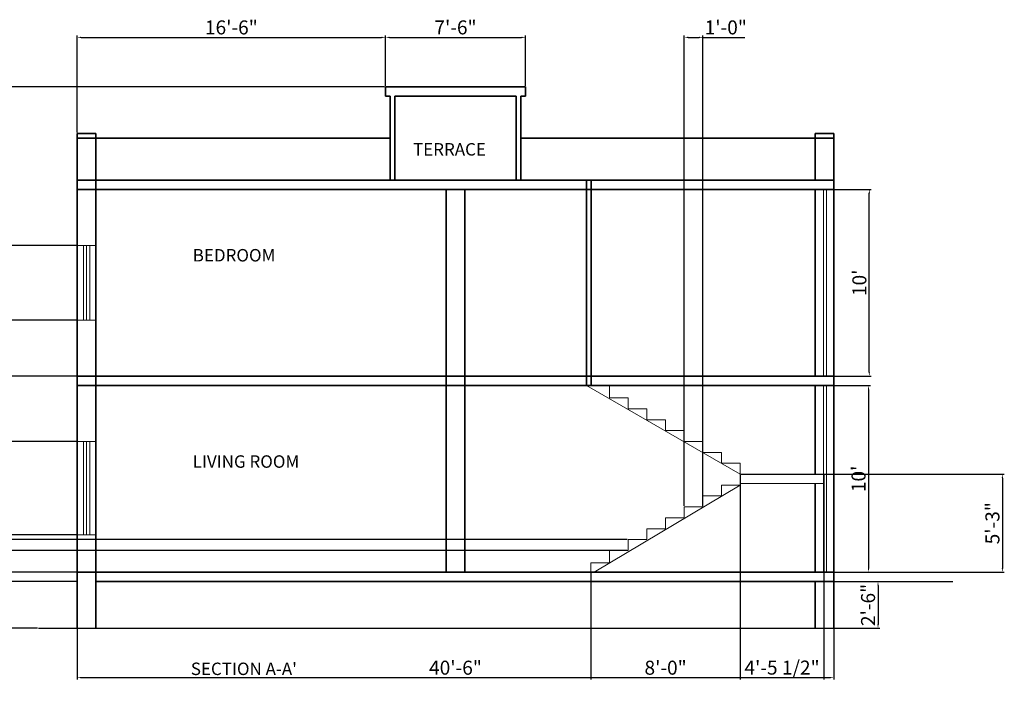
# Model space of a CAD drawing. Units: inches. Extents: x 600 to 1805, y 898 to 2057.
# Tile 4 of 5: x 1172 to 1805, y 898 to 1329. Entities that reach past the tile are written whole.
import ezdxf

# ---------------------------------------------------------------- set-up
doc = ezdxf.new("R2010")
doc.units = ezdxf.units.IN
for name, color, linetype, lineweight in [('A-ANNO-DIMS', 2, 'Continuous', 18), ('A-ANNO-TEXT', 7, 'Continuous', 25), ('A-AREA-IDEN', 7, 'Continuous', 18), ('A-FLOR-STRS', 3, 'Continuous', 20), ('A-SECT', 7, 'Continuous', 35), ('C-SITE', 7, 'Continuous', 25)]:
    doc.layers.add(name, color=color, linetype=linetype, lineweight=lineweight)
doc.layers.add('A-GLAZ', color=244, linetype='Continuous', lineweight=20, true_color=0x991b1e)
doc.styles.get("Standard").update_dxf_attribs({"font": 'arial.ttf'})
doc.dimstyles.new('ISO-25', dxfattribs={"dimtxt": 9, "dimasz": 2.5, "dimexe": 1.25, "dimexo": 0.625, "dimtad": 1, "dimlunit": 3, "dimtxsty": 'Standard', "dimcen": 2.5, "dimadec": 0, "dimazin": 0, "dimtfac": 1, "dimtmove": 0, "dimatfit": 3, "dimfxl": 1, "dimarcsym": 0})

# ---------------------------------------------------------------- blocks, each defined once
blk = doc.blocks.new('*D15')
at = {"layer": 'A-ANNO-DIMS', "color": 0, "lineweight": -2, "transparency": 16777216}
for p, q in [((1717.22, 967.8), (1725.05, 967.8)), ((1723.8, 965.3), (1723.8, 940.3)), ((1717.22, 937.8), (1725.05, 937.8))]:
    blk.add_line(p, q, dxfattribs=at)
at = {"layer": 'A-ANNO-DIMS', "color": 0, "transparency": 16777216}
for points in [[(1723.38, 965.3), (1724.21, 965.3), (1723.8, 967.8)], [(1723.38, 940.3), (1724.21, 940.3), (1723.8, 937.8)]]:
    blk.add_solid(points, dxfattribs=at)
at = {"layer": 'Defpoints', "color": 0, "transparency": 16777216}
for p in [(1716.6, 967.8), (1716.6, 937.8), (1723.8, 937.8)]:
    blk.add_point(p, dxfattribs=at)
at = {"layer": 'A-ANNO-DIMS', "color": 0, "transparency": 16777216, "insert": (1718.58, 952.8), "char_height": 9, "attachment_point": 5, "rotation": 90}
blk.add_mtext('2\'-6"', dxfattribs=at)
blk = doc.blocks.new('*D16')
at = {"layer": 'A-ANNO-DIMS', "color": 0, "lineweight": -2, "transparency": 16777216}
for p, q in [((1690.45, 1093.8), (1718.92, 1093.8)), ((1717.67, 1091.3), (1717.67, 976.3)), ((1690.45, 973.8), (1718.92, 973.8))]:
    blk.add_line(p, q, dxfattribs=at)
at = {"layer": 'A-ANNO-DIMS', "color": 0, "transparency": 16777216}
for points in [[(1717.25, 1091.3), (1718.09, 1091.3), (1717.67, 1093.8)], [(1717.25, 976.3), (1718.09, 976.3), (1717.67, 973.8)]]:
    blk.add_solid(points, dxfattribs=at)
at = {"layer": 'Defpoints', "color": 0, "transparency": 16777216}
for p in [(1689.82, 1093.8), (1689.82, 973.8), (1717.67, 973.8)]:
    blk.add_point(p, dxfattribs=at)
at = {"layer": 'A-ANNO-DIMS', "color": 0, "transparency": 16777216, "insert": (1712.45, 1033.8), "char_height": 9, "attachment_point": 5, "rotation": 90}
blk.add_mtext("10'", dxfattribs=at)
blk = doc.blocks.new('*D17')
at = {"layer": 'A-ANNO-DIMS', "color": 0, "lineweight": -2, "transparency": 16777216}
for p, q in [((1689.39, 1219.8), (1719.47, 1219.8)), ((1718.22, 1102.3), (1718.22, 1217.3)), ((1689.39, 1099.8), (1719.47, 1099.8))]:
    blk.add_line(p, q, dxfattribs=at)
at = {"layer": 'A-ANNO-DIMS', "color": 0, "transparency": 16777216}
for points in [[(1717.8, 1217.3), (1718.64, 1217.3), (1718.22, 1219.8)], [(1717.8, 1102.3), (1718.64, 1102.3), (1718.22, 1099.8)]]:
    blk.add_solid(points, dxfattribs=at)
at = {"layer": 'Defpoints', "color": 0, "transparency": 16777216}
for p in [(1688.76, 1219.8), (1718.22, 1219.8), (1688.76, 1099.8)]:
    blk.add_point(p, dxfattribs=at)
at = {"layer": 'A-ANNO-DIMS', "color": 0, "transparency": 16777216, "insert": (1713, 1159.8), "char_height": 9, "attachment_point": 5, "rotation": 90}
blk.add_mtext("10'", dxfattribs=at)
blk = doc.blocks.new('*D41')
at = {"layer": 'A-ANNO-DIMS', "color": 0, "lineweight": -2, "transparency": 16777216}
for p, q in [((1209.34, 937.18), (1209.34, 904.83)), ((1695.34, 937.18), (1695.34, 904.83)), ((1211.84, 906.08), (1692.84, 906.08))]:
    blk.add_line(p, q, dxfattribs=at)
at = {"layer": 'A-ANNO-DIMS', "color": 0, "transparency": 16777216}
for points in [[(1211.84, 906.49), (1211.84, 905.66), (1209.34, 906.08)], [(1692.84, 906.49), (1692.84, 905.66), (1695.34, 906.08)]]:
    blk.add_solid(points, dxfattribs=at)
at = {"layer": 'Defpoints', "color": 0, "transparency": 16777216}
for p in [(1209.34, 937.8), (1695.34, 937.8), (1695.34, 906.08)]:
    blk.add_point(p, dxfattribs=at)
at = {"layer": 'A-ANNO-DIMS', "color": 0, "transparency": 16777216, "insert": (1452.34, 911.3), "char_height": 9, "attachment_point": 5}
blk.add_mtext('40\'-6"', dxfattribs=at)
blk = doc.blocks.new('*D42')
at = {"layer": 'A-ANNO-DIMS', "color": 0, "lineweight": -2, "transparency": 16777216}
for p, q in [((1406.71, 1285.8), (1106.33, 1285.8)), ((1107.58, 940.3), (1107.58, 1283.3)), ((1183.78, 937.8), (1106.33, 937.8))]:
    blk.add_line(p, q, dxfattribs=at)
at = {"layer": 'A-ANNO-DIMS', "color": 0, "transparency": 16777216}
for points in [[(1107.16, 1283.3), (1107.99, 1283.3), (1107.58, 1285.8)], [(1107.16, 940.3), (1107.99, 940.3), (1107.58, 937.8)]]:
    blk.add_solid(points, dxfattribs=at)
at = {"layer": 'Defpoints', "color": 0, "transparency": 16777216}
for p in [(1107.58, 1285.8), (1407.34, 1285.8), (1184.4, 937.8)]:
    blk.add_point(p, dxfattribs=at)
at = {"layer": 'A-ANNO-DIMS', "color": 0, "transparency": 16777216, "insert": (1102.36, 1111.8), "char_height": 9, "attachment_point": 5, "rotation": 90}
blk.add_mtext('29\'-0"', dxfattribs=at)
blk = doc.blocks.new('*D43')
at = {"layer": 'A-ANNO-DIMS', "color": 0, "lineweight": -2, "transparency": 16777216}
for p, q in [((1635.34, 1036.18), (1635.34, 904.83)), ((1539.34, 973.18), (1539.34, 904.83)), ((1541.84, 906.08), (1632.84, 906.08))]:
    blk.add_line(p, q, dxfattribs=at)
at = {"layer": 'A-ANNO-DIMS', "color": 0, "transparency": 16777216}
for points in [[(1541.84, 906.49), (1541.84, 905.66), (1539.34, 906.08)], [(1632.84, 906.49), (1632.84, 905.66), (1635.34, 906.08)]]:
    blk.add_solid(points, dxfattribs=at)
at = {"layer": 'Defpoints', "color": 0, "transparency": 16777216}
for p in [(1635.34, 1036.8), (1539.34, 973.8), (1635.34, 906.08)]:
    blk.add_point(p, dxfattribs=at)
at = {"layer": 'A-ANNO-DIMS', "color": 0, "transparency": 16777216, "insert": (1587.34, 911.3), "char_height": 9, "attachment_point": 5}
blk.add_mtext('8\'-0"', dxfattribs=at)
blk = doc.blocks.new('*D44')
at = {"layer": 'A-ANNO-DIMS', "color": 0, "lineweight": -2, "transparency": 16777216}
for p, q in [((1635.34, 1036.18), (1635.34, 904.83)), ((1688.95, 1036.18), (1688.95, 904.83)), ((1637.84, 906.08), (1686.45, 906.08))]:
    blk.add_line(p, q, dxfattribs=at)
at = {"layer": 'A-ANNO-DIMS', "color": 0, "transparency": 16777216}
for points in [[(1637.84, 906.49), (1637.84, 905.66), (1635.34, 906.08)], [(1686.45, 906.49), (1686.45, 905.66), (1688.95, 906.08)]]:
    blk.add_solid(points, dxfattribs=at)
at = {"layer": 'Defpoints', "color": 0, "transparency": 16777216}
for p in [(1635.34, 1036.8), (1688.95, 1036.8), (1688.95, 906.08)]:
    blk.add_point(p, dxfattribs=at)
at = {"layer": 'A-ANNO-DIMS', "color": 0, "transparency": 16777216, "insert": (1662.14, 911.36), "char_height": 9, "attachment_point": 5}
blk.add_mtext('4\'-5 1/2"', dxfattribs=at)
blk = doc.blocks.new('*D45')
at = {"layer": 'A-ANNO-DIMS', "color": 0, "lineweight": -2, "transparency": 16777216}
for p, q in [((1635.96, 1036.8), (1804.94, 1036.8)), ((1803.69, 1034.3), (1803.69, 976.3)), ((1539.96, 973.8), (1804.94, 973.8))]:
    blk.add_line(p, q, dxfattribs=at)
at = {"layer": 'A-ANNO-DIMS', "color": 0, "transparency": 16777216}
for points in [[(1803.28, 1034.3), (1804.11, 1034.3), (1803.69, 1036.8)], [(1803.28, 976.3), (1804.11, 976.3), (1803.69, 973.8)]]:
    blk.add_solid(points, dxfattribs=at)
at = {"layer": 'Defpoints', "color": 0, "transparency": 16777216}
for p in [(1635.34, 1036.8), (1539.34, 973.8), (1803.69, 973.8)]:
    blk.add_point(p, dxfattribs=at)
at = {"layer": 'A-ANNO-DIMS', "color": 0, "transparency": 16777216, "insert": (1798.47, 1005.3), "char_height": 9, "attachment_point": 5, "rotation": 90}
blk.add_mtext('5\'-3"', dxfattribs=at)
blk = doc.blocks.new('*D46')
at = {"layer": 'A-ANNO-DIMS', "color": 0, "lineweight": -2, "transparency": 16777216}
for p, q in [((1599.34, 1016.43), (1599.34, 1318.78)), ((1601.84, 1317.53), (1608.84, 1317.53)), ((1611.34, 1016.43), (1611.34, 1318.78)), ((1611.34, 1317.53), (1638.16, 1317.53))]:
    blk.add_line(p, q, dxfattribs=at)
at = {"layer": 'A-ANNO-DIMS', "color": 0, "transparency": 16777216}
for points in [[(1601.84, 1317.94), (1601.84, 1317.11), (1599.34, 1317.53)], [(1608.84, 1317.94), (1608.84, 1317.11), (1611.34, 1317.53)]]:
    blk.add_solid(points, dxfattribs=at)
at = {"layer": 'Defpoints', "color": 0, "transparency": 16777216}
for p in [(1611.34, 1317.53), (1599.34, 1015.8), (1611.34, 1015.8)]:
    blk.add_point(p, dxfattribs=at)
at = {"layer": 'A-ANNO-DIMS', "color": 0, "transparency": 16777216, "insert": (1626, 1322.75), "char_height": 9, "attachment_point": 5}
blk.add_mtext('1\'-0"', dxfattribs=at)
blk = doc.blocks.new('*D47')
at = {"layer": 'A-ANNO-DIMS', "color": 0, "lineweight": -2, "transparency": 16777216}
for p, q in [((1107.58, 994.8), (1107.58, 1022.48)), ((1562.71, 994.8), (1106.33, 994.8)), ((1562.71, 987.8), (1106.33, 987.8)), ((1107.58, 990.3), (1107.58, 992.3))]:
    blk.add_line(p, q, dxfattribs=at)
at = {"layer": 'A-ANNO-DIMS', "color": 0, "transparency": 16777216}
for points in [[(1107.16, 992.3), (1107.99, 992.3), (1107.58, 994.8)], [(1107.16, 990.3), (1107.99, 990.3), (1107.58, 987.8)]]:
    blk.add_solid(points, dxfattribs=at)
at = {"layer": 'Defpoints', "color": 0, "transparency": 16777216}
for p in [(1107.58, 994.8), (1563.34, 994.8), (1563.34, 987.8)]:
    blk.add_point(p, dxfattribs=at)
at = {"layer": 'A-ANNO-DIMS', "color": 0, "transparency": 16777216, "insert": (1102.36, 1009.89), "char_height": 9, "attachment_point": 5, "rotation": 90}
blk.add_mtext('0\'-7"', dxfattribs=at)
blk = doc.blocks.new('*D48')
at = {"layer": 'A-ANNO-DIMS', "color": 0, "lineweight": -2, "transparency": 16777216}
for p, q in [((1407.34, 1286.43), (1407.34, 1318.78)), ((1409.84, 1317.53), (1494.84, 1317.53)), ((1497.34, 1286.43), (1497.34, 1318.78))]:
    blk.add_line(p, q, dxfattribs=at)
at = {"layer": 'A-ANNO-DIMS', "color": 0, "transparency": 16777216}
for points in [[(1409.84, 1317.94), (1409.84, 1317.11), (1407.34, 1317.53)], [(1494.84, 1317.94), (1494.84, 1317.11), (1497.34, 1317.53)]]:
    blk.add_solid(points, dxfattribs=at)
at = {"layer": 'Defpoints', "color": 0, "transparency": 16777216}
for p in [(1497.34, 1317.53), (1407.34, 1285.8), (1497.34, 1285.8)]:
    blk.add_point(p, dxfattribs=at)
at = {"layer": 'A-ANNO-DIMS', "color": 0, "transparency": 16777216, "insert": (1452.34, 1322.75), "char_height": 9, "attachment_point": 5}
blk.add_mtext('7\'-6"', dxfattribs=at)
blk = doc.blocks.new('*D49')
at = {"layer": 'A-ANNO-DIMS', "color": 0, "lineweight": -2, "transparency": 16777216}
for p, q in [((1209.34, 1256.43), (1209.34, 1318.78)), ((1211.84, 1317.53), (1404.84, 1317.53)), ((1407.34, 1286.43), (1407.34, 1318.78))]:
    blk.add_line(p, q, dxfattribs=at)
at = {"layer": 'A-ANNO-DIMS', "color": 0, "transparency": 16777216}
for points in [[(1211.84, 1317.94), (1211.84, 1317.11), (1209.34, 1317.53)], [(1404.84, 1317.94), (1404.84, 1317.11), (1407.34, 1317.53)]]:
    blk.add_solid(points, dxfattribs=at)
at = {"layer": 'Defpoints', "color": 0, "transparency": 16777216}
for p in [(1407.34, 1317.53), (1407.34, 1285.8), (1209.34, 1255.8)]:
    blk.add_point(p, dxfattribs=at)
at = {"layer": 'A-ANNO-DIMS', "color": 0, "transparency": 16777216, "insert": (1308.34, 1322.75), "char_height": 9, "attachment_point": 5}
blk.add_mtext('16\'-6"', dxfattribs=at)
blk = doc.blocks.new('*D50')
at = {"layer": 'A-ANNO-DIMS', "color": 0, "lineweight": -2, "transparency": 16777216}
for p, q in [((1107.58, 997.8), (1107.58, 1025.63)), ((1208.71, 997.8), (1106.33, 997.8)), ((1107.58, 976.3), (1107.58, 995.3)), ((1208.71, 973.8), (1106.33, 973.8))]:
    blk.add_line(p, q, dxfattribs=at)
at = {"layer": 'A-ANNO-DIMS', "color": 0, "transparency": 16777216}
for points in [[(1107.16, 995.3), (1107.99, 995.3), (1107.58, 997.8)], [(1107.16, 976.3), (1107.99, 976.3), (1107.58, 973.8)]]:
    blk.add_solid(points, dxfattribs=at)
at = {"layer": 'Defpoints', "color": 0, "transparency": 16777216}
for p in [(1107.58, 997.8), (1209.34, 997.8), (1209.34, 973.8)]:
    blk.add_point(p, dxfattribs=at)
at = {"layer": 'A-ANNO-DIMS', "color": 0, "transparency": 16777216, "insert": (1102.36, 1012.97), "char_height": 9, "attachment_point": 5, "rotation": 90}
blk.add_mtext('2\'-0"', dxfattribs=at)
blk = doc.blocks.new('*D51')
at = {"layer": 'A-ANNO-DIMS', "color": 0, "lineweight": -2, "transparency": 16777216}
for p, q in [((1208.71, 1057.8), (1106.33, 1057.8)), ((1107.58, 1000.3), (1107.58, 1055.3)), ((1208.71, 997.8), (1106.33, 997.8))]:
    blk.add_line(p, q, dxfattribs=at)
at = {"layer": 'A-ANNO-DIMS', "color": 0, "transparency": 16777216}
for points in [[(1107.16, 1055.3), (1107.99, 1055.3), (1107.58, 1057.8)], [(1107.16, 1000.3), (1107.99, 1000.3), (1107.58, 997.8)]]:
    blk.add_solid(points, dxfattribs=at)
at = {"layer": 'Defpoints', "color": 0, "transparency": 16777216}
for p in [(1107.58, 1057.8), (1209.34, 1057.8), (1209.34, 997.8)]:
    blk.add_point(p, dxfattribs=at)
at = {"layer": 'A-ANNO-DIMS', "color": 0, "transparency": 16777216, "insert": (1102.36, 1027.8), "char_height": 9, "attachment_point": 5, "rotation": 90}
blk.add_mtext('5\'-0"', dxfattribs=at)
blk = doc.blocks.new('*D52')
at = {"layer": 'A-ANNO-DIMS', "color": 0, "lineweight": -2, "transparency": 16777216}
for p, q in [((1208.71, 1135.8), (1106.33, 1135.8)), ((1107.58, 1102.3), (1107.58, 1133.3)), ((1208.71, 1099.8), (1106.33, 1099.8))]:
    blk.add_line(p, q, dxfattribs=at)
at = {"layer": 'A-ANNO-DIMS', "color": 0, "transparency": 16777216}
for points in [[(1107.16, 1133.3), (1107.99, 1133.3), (1107.58, 1135.8)], [(1107.16, 1102.3), (1107.99, 1102.3), (1107.58, 1099.8)]]:
    blk.add_solid(points, dxfattribs=at)
at = {"layer": 'Defpoints', "color": 0, "transparency": 16777216}
for p in [(1107.58, 1135.8), (1209.34, 1135.8), (1209.34, 1099.8)]:
    blk.add_point(p, dxfattribs=at)
at = {"layer": 'A-ANNO-DIMS', "color": 0, "transparency": 16777216, "insert": (1102.35, 1117.8), "char_height": 9, "attachment_point": 5, "rotation": 90}
blk.add_mtext('3\'-0"', dxfattribs=at)
blk = doc.blocks.new('*D53')
at = {"layer": 'A-ANNO-DIMS', "color": 0, "lineweight": -2, "transparency": 16777216}
for p, q in [((1208.71, 1183.8), (1106.33, 1183.8)), ((1107.58, 1138.3), (1107.58, 1181.3)), ((1208.71, 1135.8), (1106.33, 1135.8))]:
    blk.add_line(p, q, dxfattribs=at)
at = {"layer": 'A-ANNO-DIMS', "color": 0, "transparency": 16777216}
for points in [[(1107.16, 1181.3), (1107.99, 1181.3), (1107.58, 1183.8)], [(1107.16, 1138.3), (1107.99, 1138.3), (1107.58, 1135.8)]]:
    blk.add_solid(points, dxfattribs=at)
at = {"layer": 'Defpoints', "color": 0, "transparency": 16777216}
for p in [(1107.58, 1183.8), (1209.34, 1183.8), (1209.34, 1135.8)]:
    blk.add_point(p, dxfattribs=at)
at = {"layer": 'A-ANNO-DIMS', "color": 0, "transparency": 16777216, "insert": (1102.36, 1159.8), "char_height": 9, "attachment_point": 5, "rotation": 90}
blk.add_mtext('4\'-0"', dxfattribs=at)

msp = doc.modelspace()

# ---------------------------------------------------------------- linework, layer by layer
at = {"layer": 'A-FLOR-STRS'}
for p, q in [((1635.337, 1036.803), (1536.421, 1093.803)), ((1551.337, 1085.803), (1551.337, 1093.803)), ((1563.337, 1085.803), (1551.337, 1085.803)), ((1563.337, 1078.803), (1563.337, 1085.803)), ((1575.337, 1078.803), (1563.337, 1078.803)), ((1575.337, 1071.803), (1575.337, 1078.803)), ((1587.337, 1071.803), (1575.337, 1071.803)), ((1587.337, 1064.803), (1587.337, 1071.803)), ((1599.337, 1064.803), (1587.337, 1064.803)), ((1599.337, 1057.803), (1599.337, 1064.803)), ((1611.337, 1057.803), (1599.337, 1057.803)), ((1611.337, 1050.803), (1611.337, 1057.803)), ((1623.337, 1050.803), (1611.337, 1050.803)), ((1623.337, 1043.803), (1623.337, 1050.803)), ((1635.337, 1043.803), (1623.337, 1043.803)), ((1635.337, 1036.803), (1635.337, 1043.803)), ((1647.337, 1036.803), (1635.337, 1036.803)), ((1635.337, 1036.803), (1635.337, 1029.803)), ((1647.337, 1036.803), (1635.337, 1036.803)), ((1688.953, 1036.803), (1647.337, 1036.803)), ((1688.953, 1030.803), (1688.953, 1036.803)), ((1635.337, 1029.803), (1541.375, 973.803)), ((1635.337, 1029.803), (1623.337, 1029.803)), ((1623.337, 1029.803), (1623.337, 1022.803)), ((1688.953, 1030.803), (1635.337, 1030.803)), ((1623.337, 1022.803), (1611.337, 1022.803)), ((1611.337, 1022.803), (1611.337, 1015.803)), ((1611.337, 1015.803), (1599.337, 1015.803)), ((1599.337, 1015.803), (1599.337, 1008.803)), ((1599.337, 1008.803), (1587.337, 1008.803)), ((1587.337, 1008.803), (1587.337, 1001.803)), ((1587.337, 1001.803), (1575.337, 1001.803)), ((1575.337, 1001.803), (1575.337, 994.803)), ((1575.337, 994.803), (1563.337, 994.803)), ((1563.337, 994.803), (1563.337, 987.803)), ((1563.337, 987.803), (1551.337, 987.803)), ((1551.337, 987.803), (1551.337, 979.803)), ((1551.337, 979.803), (1539.337, 979.803)), ((1539.337, 979.803), (1539.337, 973.803))]:
    msp.add_line(p, q, dxfattribs=at)
at = {"layer": 'A-GLAZ'}
for p, q in [((1688.765, 1219.803), (1688.765, 1099.803)), ((1690.765, 1219.803), (1690.765, 1099.803)), ((1221.337, 1183.803), (1209.337, 1183.803)), ((1213.337, 1183.803), (1213.337, 1135.803)), ((1215.337, 1183.803), (1215.337, 1135.803)), ((1217.337, 1183.803), (1217.337, 1135.803)), ((1221.337, 1135.803), (1209.337, 1135.803)), ((1688.765, 1093.803), (1688.765, 973.803)), ((1690.765, 1093.803), (1690.765, 973.803)), ((1221.337, 1057.803), (1209.337, 1057.803)), ((1213.337, 1057.803), (1213.337, 997.803)), ((1215.337, 1057.803), (1215.337, 997.803)), ((1217.337, 1057.803), (1217.337, 997.803)), ((1221.337, 997.803), (1209.337, 997.803))]:
    msp.add_line(p, q, dxfattribs=at)
at = {"layer": 'A-SECT'}
for p, q in [((1497.337, 1285.803), (1407.337, 1285.803)), ((1407.337, 1279.803), (1407.337, 1285.803)), ((1497.337, 1279.803), (1497.337, 1285.803)), ((1410.337, 1279.803), (1407.337, 1279.803)), ((1410.337, 1225.803), (1410.337, 1279.803)), ((1413.337, 1225.803), (1413.337, 1279.803)), ((1491.337, 1279.803), (1413.337, 1279.803)), ((1491.337, 1225.803), (1491.337, 1279.803)), ((1494.337, 1225.803), (1494.337, 1279.803)), ((1497.337, 1279.803), (1494.337, 1279.803)), ((1209.337, 1219.803), (1209.337, 1255.803)), ((1209.337, 1255.803), (1221.337, 1255.803)), ((1209.337, 1252.803), (1410.337, 1252.803)), ((1221.337, 1225.803), (1221.337, 1255.803)), ((1695.337, 1252.803), (1494.337, 1252.803)), ((1683.337, 1225.803), (1683.337, 1255.803)), ((1695.337, 1255.803), (1683.337, 1255.803)), ((1695.337, 1219.803), (1695.337, 1255.803)), ((1221.337, 1225.803), (1209.337, 1225.803)), ((1695.337, 1225.803), (1221.337, 1225.803)), ((1221.337, 1093.803), (1221.337, 1225.803)), ((1536.421, 1093.803), (1536.421, 1225.803)), ((1539.421, 1093.803), (1539.421, 1225.803)), ((1209.337, 1093.803), (1209.337, 1219.803)), ((1221.337, 1219.803), (1209.337, 1219.803)), ((1695.337, 1219.803), (1221.337, 1219.803)), ((1446.337, 1093.803), (1446.337, 1219.803)), ((1458.337, 1093.803), (1458.337, 1219.803)), ((1683.337, 1099.803), (1683.337, 1219.803)), ((1695.337, 1093.803), (1695.337, 1219.803)), ((1221.337, 1099.803), (1209.337, 1099.803)), ((1695.337, 1099.803), (1221.337, 1099.803)), ((1209.337, 967.803), (1209.337, 1093.803)), ((1221.337, 1093.803), (1209.337, 1093.803)), ((1695.337, 1093.803), (1221.337, 1093.803)), ((1221.337, 973.803), (1221.337, 1093.803)), ((1446.337, 973.803), (1446.337, 1093.803)), ((1458.337, 973.803), (1458.337, 1093.803)), ((1683.337, 1036.803), (1683.337, 1093.803)), ((1695.337, 967.803), (1695.337, 1093.803)), ((1683.337, 973.803), (1683.337, 1030.803)), ((1221.337, 973.803), (1209.337, 973.803)), ((1695.337, 973.803), (1221.337, 973.803)), ((1221.337, 937.803), (1221.337, 973.803)), ((1209.337, 937.803), (1209.337, 967.803)), ((1695.337, 967.803), (1221.337, 967.803)), ((1683.337, 937.803), (1683.337, 967.803)), ((1695.337, 937.803), (1695.337, 967.803))]:
    msp.add_line(p, q, dxfattribs=at)
at = {"layer": 'C-SITE'}
for p, q in [((1209.337, 967.803), (1139.301, 967.803)), ((1695.337, 967.803), (1771.97, 967.803)), ((1184.402, 937.803), (1723.796, 937.803))]:
    msp.add_line(p, q, dxfattribs=at)

# ---------------------------------------------------------------- texts
at = {"layer": 'A-ANNO-TEXT', "insert": (1282.294, 915.743), "char_height": 8, "attachment_point": 1}
msp.add_mtext_dynamic_manual_height_columns("SECTION A-A'", width=74.76978, gutter_width=12.5, heights=[0], dxfattribs=at)
at = {"layer": 'A-AREA-IDEN', "char_height": 8, "attachment_point": 1}
for s, width, insert in [('TERRACE ', 58.88863, (1425.055, 1249.576)), ('BEDROOM ', 58.88863, (1283.53, 1181.511)), ('LIVING ROOM', 75.00689, (1283.53, 1048.943))]:
    msp.add_mtext_dynamic_manual_height_columns(s, width=width, gutter_width=12.5, heights=[0], dxfattribs=dict(at, insert=insert))

# ---------------------------------------------------------------- dimensions: what is measured, and where the dimension line sits
at = {"layer": 'A-ANNO-DIMS'}
for base, p1, p2, picture, middle in [((1407.337, 1317.528), (1209.337, 1255.803), (1407.337, 1285.803), '*D49', (1308.337, 1322.748)), ((1497.337, 1317.528), (1407.337, 1285.803), (1497.337, 1285.803), '*D48', (1452.337, 1322.748)), ((1611.337, 1317.528), (1599.337, 1015.803), (1611.337, 1015.803), '*D46', (1626.001, 1322.748)), ((1635.337, 906.078), (1539.337, 973.803), (1635.337, 1036.803), '*D43', (1587.337, 911.298)), ((1688.953, 906.078), (1635.337, 1036.803), (1688.953, 1036.803), '*D44', (1662.145, 911.356)), ((1695.337, 906.078), (1209.337, 937.803), (1695.337, 937.803), '*D41', (1452.337, 911.298))]:
    dim = msp.add_linear_dim(base=base, p1=p1, p2=p2, dimstyle='ISO-25', override={"dimdec": 1, "dimlfac": 1, "dimrnd": 0, "dimzin": 1, "dimdsep": 46, "dimlunit": 4, "dimfrac": 2}, dxfattribs=at)
    dim.commit()
    dim.dimension.update_dxf_attribs({"geometry": picture, "text_midpoint": middle})
for base, p1, p2, override, picture, middle in [((1107.576, 1285.803), (1184.402, 937.803), (1407.337, 1285.803), {"dimdec": 1, "dimlfac": 1, "dimrnd": 0, "dimzin": 1, "dimdsep": 46, "dimlunit": 4, "dimfrac": 2}, '*D42', (1102.356, 1111.803)), ((1718.22, 1219.803), (1688.765, 1099.803), (1688.765, 1219.803), {"dimclrd": 0, "dimclre": 0, "dimclrt": 0}, '*D17', (1713, 1159.803)), ((1107.576, 1183.803), (1209.337, 1135.803), (1209.337, 1183.803), {"dimdec": 1, "dimlfac": 1, "dimrnd": 0, "dimzin": 1, "dimdsep": 46, "dimlunit": 4, "dimfrac": 2}, '*D53', (1102.356, 1159.803)), ((1107.576, 1135.803), (1209.337, 1099.803), (1209.337, 1135.803), {"dimdec": 1, "dimlfac": 1, "dimrnd": 0, "dimzin": 1, "dimdsep": 46, "dimlunit": 4, "dimfrac": 2}, '*D52', (1102.353, 1117.803)), ((1717.67, 973.803), (1689.821, 1093.803), (1689.821, 973.803), {"dimclrd": 0, "dimclre": 0, "dimclrt": 0}, '*D16', (1712.449, 1033.803)), ((1107.576, 1057.803), (1209.337, 997.803), (1209.337, 1057.803), {"dimdec": 1, "dimlfac": 1, "dimrnd": 0, "dimzin": 1, "dimdsep": 46, "dimlunit": 4, "dimfrac": 2}, '*D51', (1102.356, 1027.803)), ((1803.695, 973.803), (1635.337, 1036.803), (1539.337, 973.803), {"dimdec": 1, "dimlfac": 1, "dimrnd": 0, "dimzin": 1, "dimdsep": 46, "dimlunit": 4, "dimfrac": 2}, '*D45', (1798.472, 1005.303)), ((1107.576, 997.803), (1209.337, 973.803), (1209.337, 997.803), {"dimdec": 1, "dimlfac": 1, "dimrnd": 0, "dimzin": 1, "dimdsep": 46, "dimlunit": 4, "dimfrac": 2}, '*D50', (1102.356, 1012.967)), ((1107.576, 994.803), (1563.337, 987.803), (1563.337, 994.803), {"dimdec": 1, "dimlfac": 1, "dimrnd": 0, "dimzin": 1, "dimdsep": 46, "dimlunit": 4, "dimfrac": 2}, '*D47', (1102.356, 1009.89)), ((1723.796, 937.803), (1716.599, 967.803), (1716.599, 937.803), {"dimclrd": 0, "dimclre": 0, "dimclrt": 0}, '*D15', (1718.576, 952.803))]:
    dim = msp.add_linear_dim(base=base, p1=p1, p2=p2, angle=90, dimstyle='ISO-25', override=override, dxfattribs=at)
    dim.commit()
    dim.dimension.update_dxf_attribs({"geometry": picture, "text_midpoint": middle})

doc.saveas('drawing.dxf')
